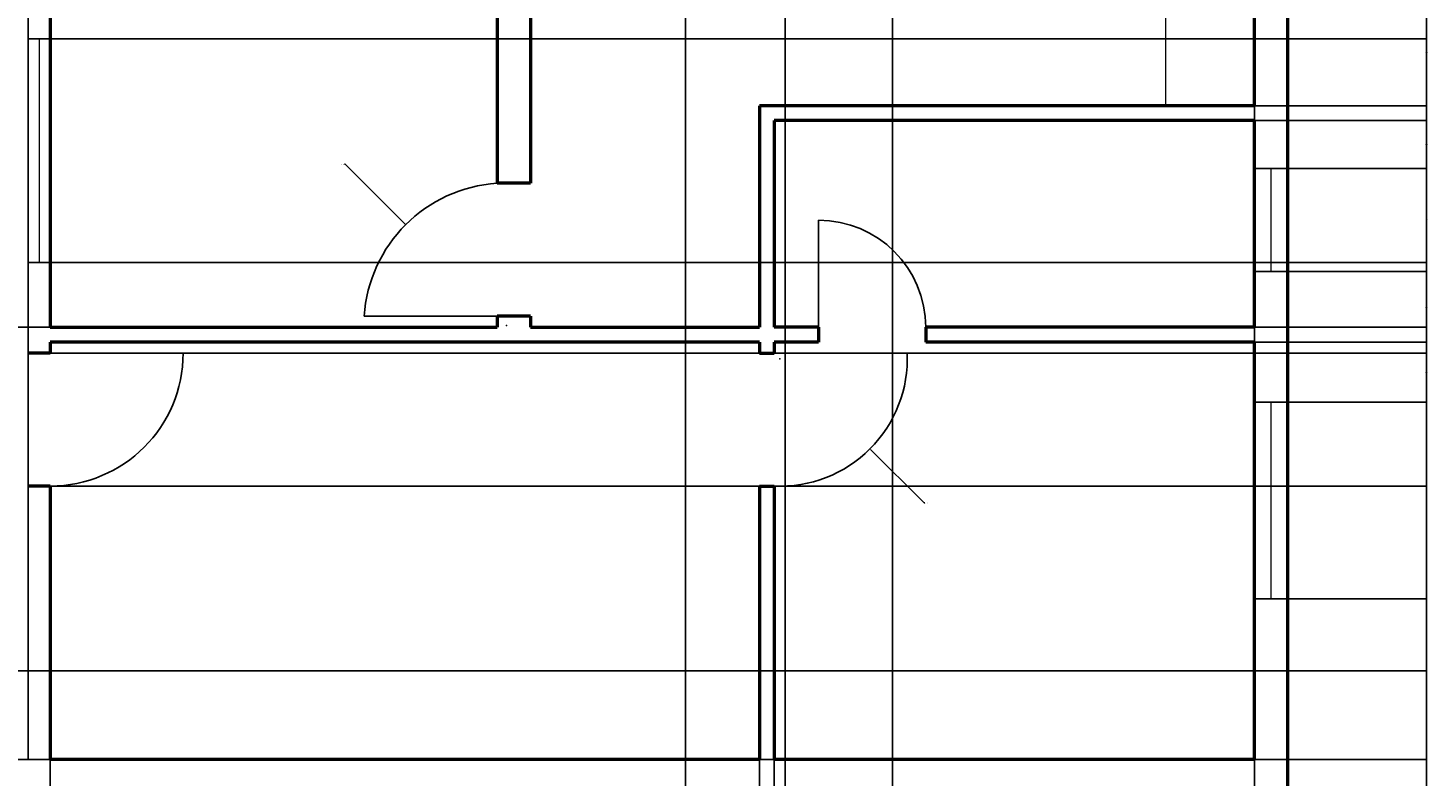
# Model space of a CAD drawing. Units: inches. Extents: x 2479 to 3284, y 2154 to 2936.
# Tile 7 of 8: x 2905 to 3284, y 2538 to 2741. Entities that reach past the tile are written whole.
import ezdxf

# ---------------------------------------------------------------- set-up
doc = ezdxf.new("R2010")
doc.units = ezdxf.units.IN
for name, color, linetype, lineweight in [('A-ANNO-DIMS', 2, 'Continuous', 18), ('A-DOOR', 3, 'Continuous', 25), ('A-FLOR-CASE', 8, 'Continuous', 18), ('A-GLAZ', 4, 'Continuous', 18), ('A-WALL', 7, 'Continuous', 50)]:
    doc.layers.add(name, color=color, linetype=linetype, lineweight=lineweight)
doc.styles.get("Standard").update_dxf_attribs({"font": 'arial.ttf'})
doc.dimstyles.get("Standard").update_dxf_attribs({"dimtxt": 0.18, "dimasz": 0.18, "dimexe": 0.18, "dimexo": 0.0625, "dimgap": 0.09, "dimtad": 0, "dimtih": 1, "dimtoh": 1, "dimdec": 4, "dimzin": 0, "dimdsep": 46, "dimtxsty": 'Standard', "dimcen": 0.09, "dimadec": 0, "dimazin": 0, "dimtfac": 1, "dimtdec": 4, "dimtofl": 0, "dimtmove": 0, "dimatfit": 3, "dimfxl": 1, "dimtolj": 1, "dimtzin": 0, "dimarcsym": 0})

# ---------------------------------------------------------------- blocks, each defined once
blk = doc.blocks.new('DOOR-SWING-29IN')
blk.add_line((29, 0), (0, 0))
blk.add_arc((29, 0), 29, 90, 180)
blk = doc.blocks.new('DOOR-SWING-36IN')
blk.add_line((36, 0), (0, 0))
blk.add_arc((36, 0), 36, 90, 180)
blk = doc.blocks.new('*D10')
at = {"layer": 'A-ANNO-DIMS', "color": 0, "lineweight": -2, "transparency": 16777216}
for p, q in [((3246.27, 2897.74), (3283.99, 2897.74)), ((3283.81, 2897.56), (3283.81, 2715.92)), ((3283.81, 2533.92), (3283.81, 2715.56)), ((3237.27, 2533.74), (3283.99, 2533.74))]:
    blk.add_line(p, q, dxfattribs=at)
at = {"layer": 'A-ANNO-DIMS', "color": 0, "transparency": 16777216}
for points in [[(3283.78, 2897.56), (3283.84, 2897.56), (3283.81, 2897.74)], [(3283.78, 2533.92), (3283.84, 2533.92), (3283.81, 2533.74)]]:
    blk.add_solid(points, dxfattribs=at)
at = {"layer": 'Defpoints', "color": 0, "transparency": 16777216}
for p in [(3246.21, 2897.74), (3283.81, 2897.74), (3237.21, 2533.74)]:
    blk.add_point(p, dxfattribs=at)
at = {"layer": 'A-ANNO-DIMS', "color": 0, "transparency": 16777216, "insert": (3283.81, 2715.74), "char_height": 0.18, "attachment_point": 5}
blk.add_mtext('\\A1;364', dxfattribs=at)
blk = doc.blocks.new('*D11')
at = {"layer": 'A-ANNO-DIMS', "color": 0, "lineweight": -2, "transparency": 16777216}
for p, q in [((2845.21, 2542.8), (2845.21, 2935.52)), ((2845.39, 2935.34), (2874.99, 2935.34)), ((2905.03, 2935.34), (2875.43, 2935.34)), ((2905.21, 2542.8), (2905.21, 2935.52))]:
    blk.add_line(p, q, dxfattribs=at)
at = {"layer": 'A-ANNO-DIMS', "color": 0, "transparency": 16777216}
for points in [[(2845.39, 2935.37), (2845.39, 2935.31), (2845.21, 2935.34)], [(2905.03, 2935.37), (2905.03, 2935.31), (2905.21, 2935.34)]]:
    blk.add_solid(points, dxfattribs=at)
at = {"layer": 'Defpoints', "color": 0, "transparency": 16777216}
for p in [(2905.21, 2935.34), (2845.21, 2542.74), (2905.21, 2542.74)]:
    blk.add_point(p, dxfattribs=at)
at = {"layer": 'A-ANNO-DIMS', "color": 0, "transparency": 16777216, "insert": (2875.21, 2935.34), "char_height": 0.18, "attachment_point": 5}
blk.add_mtext('\\A1;60', dxfattribs=at)
blk = doc.blocks.new('*D20')
at = {"layer": 'A-ANNO-DIMS', "color": 0, "lineweight": -2, "transparency": 16777216}
for p, q in [((2911.27, 2542.74), (3283.99, 2542.74)), ((3283.81, 2542.56), (3283.81, 2538.42)), ((3283.81, 2533.92), (3283.81, 2538.06)), ((2911.27, 2533.74), (3283.99, 2533.74))]:
    blk.add_line(p, q, dxfattribs=at)
at = {"layer": 'A-ANNO-DIMS', "color": 0, "transparency": 16777216}
for points in [[(3283.78, 2542.56), (3283.84, 2542.56), (3283.81, 2542.74)], [(3283.78, 2533.92), (3283.84, 2533.92), (3283.81, 2533.74)]]:
    blk.add_solid(points, dxfattribs=at)
at = {"layer": 'Defpoints', "color": 0, "transparency": 16777216}
for p in [(2911.21, 2542.74), (3283.81, 2542.74), (2911.21, 2533.74)]:
    blk.add_point(p, dxfattribs=at)
at = {"layer": 'A-ANNO-DIMS', "color": 0, "transparency": 16777216, "insert": (3283.81, 2538.24), "char_height": 0.18, "attachment_point": 5}
blk.add_mtext('\\A1;9', dxfattribs=at)
blk = doc.blocks.new('*D21')
at = {"layer": 'A-ANNO-DIMS', "color": 0, "lineweight": -2, "transparency": 16777216}
for p, q in [((2905.27132, 2616.739749), (3283.98882, 2616.739749)), ((3283.80882, 2616.559749), (3283.80882, 2579.919749)), ((3283.80882, 2542.919749), (3283.80882, 2579.559749)), ((2911.27132, 2542.739749), (3283.98882, 2542.739749))]:
    blk.add_line(p, q, dxfattribs=at)
at = {"layer": 'A-ANNO-DIMS', "color": 0, "transparency": 16777216}
for points in [[(3283.77882, 2616.559749), (3283.83882, 2616.559749), (3283.80882, 2616.739749)], [(3283.77882, 2542.919749), (3283.83882, 2542.919749), (3283.80882, 2542.739749)]]:
    blk.add_solid(points, dxfattribs=at)
at = {"layer": 'Defpoints', "color": 0, "transparency": 16777216}
for p in [(2905.20882, 2616.739749), (3283.80882, 2616.739749), (2911.20882, 2542.739749)]:
    blk.add_point(p, dxfattribs=at)
at = {"layer": 'A-ANNO-DIMS', "color": 0, "transparency": 16777216, "insert": (3283.80882, 2579.739749), "char_height": 0.18, "attachment_point": 5}
blk.add_mtext('\\A1;74', dxfattribs=at)
blk = doc.blocks.new('*D22')
at = {"layer": 'A-ANNO-DIMS', "color": 0, "lineweight": -2, "transparency": 16777216}
for p, q in [((2905.27, 2677.32), (3283.99, 2677.32)), ((3283.81, 2677.14), (3283.81, 2665.21)), ((3283.81, 2652.92), (3283.81, 2664.85)), ((2905.27, 2652.74), (3283.99, 2652.74))]:
    blk.add_line(p, q, dxfattribs=at)
at = {"layer": 'A-ANNO-DIMS', "color": 0, "transparency": 16777216}
for points in [[(3283.78, 2677.14), (3283.84, 2677.14), (3283.81, 2677.32)], [(3283.78, 2652.92), (3283.84, 2652.92), (3283.81, 2652.74)]]:
    blk.add_solid(points, dxfattribs=at)
at = {"layer": 'Defpoints', "color": 0, "transparency": 16777216}
for p in [(2905.21, 2677.32), (3283.81, 2677.32), (2905.21, 2652.74)]:
    blk.add_point(p, dxfattribs=at)
at = {"layer": 'A-ANNO-DIMS', "color": 0, "transparency": 16777216, "insert": (3283.81, 2665.03), "char_height": 0.18, "attachment_point": 5}
blk.add_mtext('\\A1;24.575', dxfattribs=at)
blk = doc.blocks.new('*D23')
at = {"layer": 'A-ANNO-DIMS', "color": 0, "lineweight": -2, "transparency": 16777216}
for p, q in [((2905.27, 2737.84), (3283.99, 2737.84)), ((3283.81, 2737.66), (3283.81, 2707.76)), ((3283.81, 2677.5), (3283.81, 2707.39)), ((2905.27, 2677.32), (3283.99, 2677.32))]:
    blk.add_line(p, q, dxfattribs=at)
at = {"layer": 'A-ANNO-DIMS', "color": 0, "transparency": 16777216}
for points in [[(3283.78, 2737.66), (3283.84, 2737.66), (3283.81, 2737.84)], [(3283.78, 2677.5), (3283.84, 2677.5), (3283.81, 2677.32)]]:
    blk.add_solid(points, dxfattribs=at)
at = {"layer": 'Defpoints', "color": 0, "transparency": 16777216}
for p in [(2905.21, 2737.84), (3283.81, 2737.84), (2905.21, 2677.32)]:
    blk.add_point(p, dxfattribs=at)
at = {"layer": 'A-ANNO-DIMS', "color": 0, "transparency": 16777216, "insert": (3283.81, 2707.58), "char_height": 0.18, "attachment_point": 5}
blk.add_mtext('\\A1;60.52', dxfattribs=at)
blk = doc.blocks.new('*D61')
at = {"layer": 'A-ANNO-DIMS', "color": 0, "lineweight": -2, "transparency": 16777216}
for p, q in [((2595.27, 2566.74), (3283.99, 2566.74)), ((3283.81, 2566.56), (3283.81, 2554.92)), ((3283.81, 2542.92), (3283.81, 2554.56)), ((2595.27, 2542.74), (3283.99, 2542.74))]:
    blk.add_line(p, q, dxfattribs=at)
at = {"layer": 'A-ANNO-DIMS', "color": 0, "transparency": 16777216}
for points in [[(3283.78, 2566.56), (3283.84, 2566.56), (3283.81, 2566.74)], [(3283.78, 2542.92), (3283.84, 2542.92), (3283.81, 2542.74)]]:
    blk.add_solid(points, dxfattribs=at)
at = {"layer": 'Defpoints', "color": 0, "transparency": 16777216}
for p in [(2595.21, 2566.74), (3283.81, 2566.74), (2595.21, 2542.74)]:
    blk.add_point(p, dxfattribs=at)
at = {"layer": 'A-ANNO-DIMS', "color": 0, "transparency": 16777216, "insert": (3283.81, 2554.74), "char_height": 0.18, "attachment_point": 5}
blk.add_mtext('\\A1;24', dxfattribs=at)
blk = doc.blocks.new('*D74')
at = {"layer": 'A-ANNO-DIMS', "color": 0, "lineweight": -2, "transparency": 16777216}
for p, q in [((3237.27, 2586.18), (3283.99, 2586.18)), ((3283.81, 2586), (3283.81, 2564.64)), ((3283.81, 2542.92), (3283.81, 2564.28)), ((3237.27, 2542.74), (3283.99, 2542.74))]:
    blk.add_line(p, q, dxfattribs=at)
at = {"layer": 'A-ANNO-DIMS', "color": 0, "transparency": 16777216}
for points in [[(3283.78, 2586), (3283.84, 2586), (3283.81, 2586.18)], [(3283.78, 2542.92), (3283.84, 2542.92), (3283.81, 2542.74)]]:
    blk.add_solid(points, dxfattribs=at)
at = {"layer": 'Defpoints', "color": 0, "transparency": 16777216}
for p in [(3237.21, 2586.18), (3283.81, 2586.18), (3237.21, 2542.74)]:
    blk.add_point(p, dxfattribs=at)
at = {"layer": 'A-ANNO-DIMS', "color": 0, "transparency": 16777216, "insert": (3283.81, 2564.46), "char_height": 0.18, "attachment_point": 5}
blk.add_mtext('\\A1;43.44', dxfattribs=at)
blk = doc.blocks.new('*D75')
at = {"layer": 'A-ANNO-DIMS', "color": 0, "lineweight": -2, "transparency": 16777216}
for p, q in [((3237.27, 2639.44), (3283.99, 2639.44)), ((3283.81, 2639.26), (3283.81, 2612.99)), ((3283.81, 2586.36), (3283.81, 2612.62)), ((3237.27, 2586.18), (3283.99, 2586.18))]:
    blk.add_line(p, q, dxfattribs=at)
at = {"layer": 'A-ANNO-DIMS', "color": 0, "transparency": 16777216}
for points in [[(3283.78, 2639.26), (3283.84, 2639.26), (3283.81, 2639.44)], [(3283.78, 2586.36), (3283.84, 2586.36), (3283.81, 2586.18)]]:
    blk.add_solid(points, dxfattribs=at)
at = {"layer": 'Defpoints', "color": 0, "transparency": 16777216}
for p in [(3237.21, 2639.44), (3283.81, 2639.44), (3237.21, 2586.18)]:
    blk.add_point(p, dxfattribs=at)
at = {"layer": 'A-ANNO-DIMS', "color": 0, "transparency": 16777216, "insert": (3283.81, 2612.81), "char_height": 0.18, "attachment_point": 5}
blk.add_mtext('\\A1;53.26', dxfattribs=at)
blk = doc.blocks.new('*D76')
at = {"layer": 'A-ANNO-DIMS', "color": 0, "lineweight": -2, "transparency": 16777216}
for p, q in [((3237.27, 2655.74), (3283.99, 2655.74)), ((3283.81, 2655.56), (3283.81, 2647.77)), ((3283.81, 2639.62), (3283.81, 2647.41)), ((3237.27, 2639.44), (3283.99, 2639.44))]:
    blk.add_line(p, q, dxfattribs=at)
at = {"layer": 'A-ANNO-DIMS', "color": 0, "transparency": 16777216}
for points in [[(3283.78, 2655.56), (3283.84, 2655.56), (3283.81, 2655.74)], [(3283.78, 2639.62), (3283.84, 2639.62), (3283.81, 2639.44)]]:
    blk.add_solid(points, dxfattribs=at)
at = {"layer": 'Defpoints', "color": 0, "transparency": 16777216}
for p in [(3237.21, 2655.74), (3283.81, 2655.74), (3237.21, 2639.44)]:
    blk.add_point(p, dxfattribs=at)
at = {"layer": 'A-ANNO-DIMS', "color": 0, "transparency": 16777216, "insert": (3283.81, 2647.59), "char_height": 0.18, "attachment_point": 5}
blk.add_mtext('\\A1;16.305', dxfattribs=at)
blk = doc.blocks.new('*D77')
at = {"layer": 'A-ANNO-DIMS', "color": 0, "lineweight": -2, "transparency": 16777216}
for p, q in [((3237.27, 2674.89), (3283.99, 2674.89)), ((3283.81, 2674.71), (3283.81, 2667.5)), ((3283.81, 2659.92), (3283.81, 2667.13)), ((3237.27, 2659.74), (3283.99, 2659.74))]:
    blk.add_line(p, q, dxfattribs=at)
at = {"layer": 'A-ANNO-DIMS', "color": 0, "transparency": 16777216}
for points in [[(3283.78, 2674.71), (3283.84, 2674.71), (3283.81, 2674.89)], [(3283.78, 2659.92), (3283.84, 2659.92), (3283.81, 2659.74)]]:
    blk.add_solid(points, dxfattribs=at)
at = {"layer": 'Defpoints', "color": 0, "transparency": 16777216}
for p in [(3237.21, 2674.89), (3283.81, 2674.89), (3237.21, 2659.74)]:
    blk.add_point(p, dxfattribs=at)
at = {"layer": 'A-ANNO-DIMS', "color": 0, "transparency": 16777216, "insert": (3283.81, 2667.31), "char_height": 0.18, "attachment_point": 5}
blk.add_mtext('\\A1;15.15', dxfattribs=at)
blk = doc.blocks.new('*D78')
at = {"layer": 'A-ANNO-DIMS', "color": 0, "lineweight": -2, "transparency": 16777216}
for p, q in [((3237.27, 2702.73), (3283.99, 2702.73)), ((3283.81, 2702.55), (3283.81, 2688.99)), ((3283.81, 2675.07), (3283.81, 2688.63)), ((3237.27, 2674.89), (3283.99, 2674.89))]:
    blk.add_line(p, q, dxfattribs=at)
at = {"layer": 'A-ANNO-DIMS', "color": 0, "transparency": 16777216}
for points in [[(3283.78, 2702.55), (3283.84, 2702.55), (3283.81, 2702.73)], [(3283.78, 2675.07), (3283.84, 2675.07), (3283.81, 2674.89)]]:
    blk.add_solid(points, dxfattribs=at)
at = {"layer": 'Defpoints', "color": 0, "transparency": 16777216}
for p in [(3237.21, 2702.73), (3283.81, 2702.73), (3237.21, 2674.89)]:
    blk.add_point(p, dxfattribs=at)
at = {"layer": 'A-ANNO-DIMS', "color": 0, "transparency": 16777216, "insert": (3283.81, 2688.81), "char_height": 0.18, "attachment_point": 5}
blk.add_mtext('\\A1;27.837', dxfattribs=at)
blk = doc.blocks.new('*D79')
at = {"layer": 'A-ANNO-DIMS', "color": 0, "lineweight": -2, "transparency": 16777216}
for p, q in [((3237.27, 2715.74), (3283.99, 2715.74)), ((3283.81, 2715.56), (3283.81, 2709.42)), ((3283.81, 2702.91), (3283.81, 2709.05)), ((3237.27, 2702.73), (3283.99, 2702.73))]:
    blk.add_line(p, q, dxfattribs=at)
at = {"layer": 'A-ANNO-DIMS', "color": 0, "transparency": 16777216}
for points in [[(3283.78, 2715.56), (3283.84, 2715.56), (3283.81, 2715.74)], [(3283.78, 2702.91), (3283.84, 2702.91), (3283.81, 2702.73)]]:
    blk.add_solid(points, dxfattribs=at)
at = {"layer": 'Defpoints', "color": 0, "transparency": 16777216}
for p in [(3237.21, 2715.74), (3283.81, 2715.74), (3237.21, 2702.73)]:
    blk.add_point(p, dxfattribs=at)
at = {"layer": 'A-ANNO-DIMS', "color": 0, "transparency": 16777216, "insert": (3283.81, 2709.23), "char_height": 0.18, "attachment_point": 5}
blk.add_mtext('\\A1;13.013', dxfattribs=at)
blk = doc.blocks.new('*D80')
at = {"layer": 'A-ANNO-DIMS', "color": 0, "lineweight": -2, "transparency": 16777216}
for p, q in [((3237.27, 2748.61), (3283.99, 2748.61)), ((3283.81, 2748.43), (3283.81, 2734.36)), ((3283.81, 2719.92), (3283.81, 2733.99)), ((3237.27, 2719.74), (3283.99, 2719.74))]:
    blk.add_line(p, q, dxfattribs=at)
at = {"layer": 'A-ANNO-DIMS', "color": 0, "transparency": 16777216}
for points in [[(3283.78, 2748.43), (3283.84, 2748.43), (3283.81, 2748.61)], [(3283.78, 2719.92), (3283.84, 2719.92), (3283.81, 2719.74)]]:
    blk.add_solid(points, dxfattribs=at)
at = {"layer": 'Defpoints', "color": 0, "transparency": 16777216}
for p in [(3237.21, 2748.61), (3283.81, 2748.61), (3237.21, 2719.74)]:
    blk.add_point(p, dxfattribs=at)
at = {"layer": 'A-ANNO-DIMS', "color": 0, "transparency": 16777216, "insert": (3283.81, 2734.18), "char_height": 0.18, "attachment_point": 5}
blk.add_mtext('\\A1;28.874', dxfattribs=at)
blk = doc.blocks.new('*D86')
at = {"layer": 'A-ANNO-DIMS', "color": 0, "lineweight": -2, "transparency": 16777216}
for p, q in [((3041.15, 2770.74), (2479.43, 2770.74)), ((2479.61, 2770.56), (2479.61, 2715.42)), ((2479.61, 2659.92), (2479.61, 2715.06)), ((2911.15, 2659.74), (2479.43, 2659.74))]:
    blk.add_line(p, q, dxfattribs=at)
at = {"layer": 'A-ANNO-DIMS', "color": 0, "transparency": 16777216}
for points in [[(2479.58, 2770.56), (2479.64, 2770.56), (2479.61, 2770.74)], [(2479.58, 2659.92), (2479.64, 2659.92), (2479.61, 2659.74)]]:
    blk.add_solid(points, dxfattribs=at)
at = {"layer": 'Defpoints', "color": 0, "transparency": 16777216}
for p in [(2479.61, 2770.74), (3041.21, 2770.74), (2911.21, 2659.74)]:
    blk.add_point(p, dxfattribs=at)
at = {"layer": 'A-ANNO-DIMS', "color": 0, "transparency": 16777216, "insert": (2479.61, 2715.24), "char_height": 0.18, "attachment_point": 5}
blk.add_mtext('\\A1;111', dxfattribs=at)
blk = doc.blocks.new('*D87')
at = {"layer": 'A-ANNO-DIMS', "color": 0, "lineweight": -2, "transparency": 16777216}
for p, q in [((2911.21, 2542.68), (2911.21, 2153.96)), ((3103.21, 2542.68), (3103.21, 2153.96)), ((2911.39, 2154.14), (3006.93, 2154.14)), ((3103.03, 2154.14), (3007.49, 2154.14))]:
    blk.add_line(p, q, dxfattribs=at)
at = {"layer": 'A-ANNO-DIMS', "color": 0, "transparency": 16777216}
for points in [[(2911.39, 2154.17), (2911.39, 2154.11), (2911.21, 2154.14)], [(3103.03, 2154.17), (3103.03, 2154.11), (3103.21, 2154.14)]]:
    blk.add_solid(points, dxfattribs=at)
at = {"layer": 'Defpoints', "color": 0, "transparency": 16777216}
for p in [(2911.21, 2542.74), (3103.21, 2542.74), (3103.21, 2154.14)]:
    blk.add_point(p, dxfattribs=at)
at = {"layer": 'A-ANNO-DIMS', "color": 0, "transparency": 16777216, "insert": (3007.21, 2154.14), "char_height": 0.18, "attachment_point": 5}
blk.add_mtext('\\A1;192', dxfattribs=at)
blk = doc.blocks.new('*D88')
at = {"layer": 'A-ANNO-DIMS', "color": 0, "lineweight": -2, "transparency": 16777216}
for p, q in [((3107.21, 2542.68), (3107.21, 2153.96)), ((3237.21, 2542.68), (3237.21, 2153.96)), ((3107.39, 2154.14), (3171.93, 2154.14)), ((3237.03, 2154.14), (3172.49, 2154.14))]:
    blk.add_line(p, q, dxfattribs=at)
at = {"layer": 'A-ANNO-DIMS', "color": 0, "transparency": 16777216}
for points in [[(3107.39, 2154.17), (3107.39, 2154.11), (3107.21, 2154.14)], [(3237.03, 2154.17), (3237.03, 2154.11), (3237.21, 2154.14)]]:
    blk.add_solid(points, dxfattribs=at)
at = {"layer": 'Defpoints', "color": 0, "transparency": 16777216}
for p in [(3107.21, 2542.74), (3237.21, 2542.74), (3237.21, 2154.14)]:
    blk.add_point(p, dxfattribs=at)
at = {"layer": 'A-ANNO-DIMS', "color": 0, "transparency": 16777216, "insert": (3172.21, 2154.14), "char_height": 0.18, "attachment_point": 5}
blk.add_mtext('\\A1;130', dxfattribs=at)
blk = doc.blocks.new('*D131')
at = {"layer": 'A-ANNO-DIMS', "color": 0, "lineweight": -2, "transparency": 16777216}
for p, q in [((3083.21, 2407.8), (3083.21, 2935.52)), ((3083.39, 2935.34), (3096.49, 2935.34)), ((3110.03, 2935.34), (3096.93, 2935.34)), ((3110.21, 2407.8), (3110.21, 2935.52))]:
    blk.add_line(p, q, dxfattribs=at)
at = {"layer": 'A-ANNO-DIMS', "color": 0, "transparency": 16777216}
for points in [[(3083.39, 2935.37), (3083.39, 2935.31), (3083.21, 2935.34)], [(3110.03, 2935.37), (3110.03, 2935.31), (3110.21, 2935.34)]]:
    blk.add_solid(points, dxfattribs=at)
at = {"layer": 'Defpoints', "color": 0, "transparency": 16777216}
for p in [(3110.21, 2935.34), (3083.21, 2407.74), (3110.21, 2407.74)]:
    blk.add_point(p, dxfattribs=at)
at = {"layer": 'A-ANNO-DIMS', "color": 0, "transparency": 16777216, "insert": (3096.71, 2935.34), "char_height": 0.18, "attachment_point": 5}
blk.add_mtext('\\A1;27', dxfattribs=at)
blk = doc.blocks.new('*D132')
at = {"layer": 'A-ANNO-DIMS', "color": 0, "lineweight": -2, "transparency": 16777216}
for p, q in [((3139.21, 2407.8), (3139.21, 2935.52)), ((3139.39, 2935.34), (3187.99, 2935.34)), ((3237.03, 2935.34), (3188.43, 2935.34)), ((3237.21, 2407.8), (3237.21, 2935.52))]:
    blk.add_line(p, q, dxfattribs=at)
at = {"layer": 'A-ANNO-DIMS', "color": 0, "transparency": 16777216}
for points in [[(3139.39, 2935.37), (3139.39, 2935.31), (3139.21, 2935.34)], [(3237.03, 2935.37), (3237.03, 2935.31), (3237.21, 2935.34)]]:
    blk.add_solid(points, dxfattribs=at)
at = {"layer": 'Defpoints', "color": 0, "transparency": 16777216}
for p in [(3237.21, 2935.34), (3139.21, 2407.74), (3237.21, 2407.74)]:
    blk.add_point(p, dxfattribs=at)
at = {"layer": 'A-ANNO-DIMS', "color": 0, "transparency": 16777216, "insert": (3188.21, 2935.34), "char_height": 0.18, "attachment_point": 5}
blk.add_mtext('\\A1;98', dxfattribs=at)
blk = doc.blocks.new('*D133')
at = {"layer": 'A-ANNO-DIMS', "color": 0, "lineweight": -2, "transparency": 16777216}
for p, q in [((2990.87, 2703.89), (2991.05, 2703.89)), ((2991.05, 2703.89), (3007.31, 2687.64)), ((3034.64, 2660.22), (3034.82, 2660.22)), ((3034.73, 2660.13), (3034.73, 2660.31))]:
    blk.add_line(p, q, dxfattribs=at)
at = {"layer": 'A-ANNO-DIMS', "color": 0, "transparency": 16777216}
blk.add_solid([(3007.33, 2687.66), (3007.29, 2687.62), (3007.43, 2687.52)], dxfattribs=at)
at = {"layer": 'Defpoints', "color": 0, "transparency": 16777216}
for p in [(3007.43, 2687.52), (3034.73, 2660.22)]:
    blk.add_point(p, dxfattribs=at)
at = {"layer": 'A-ANNO-DIMS', "color": 0, "transparency": 16777216, "insert": (2990.32, 2703.89), "char_height": 0.18, "attachment_point": 5}
blk.add_mtext('\\A1;R38.605', dxfattribs=at)
blk = doc.blocks.new('*D134')
at = {"layer": 'A-ANNO-DIMS', "color": 0, "lineweight": -2, "transparency": 16777216}
for p, q in [((3108.62, 2651.24), (3108.8, 2651.24)), ((3108.71, 2651.15), (3108.71, 2651.33)), ((3147.78, 2612.17), (3133.26, 2626.69)), ((3147.96, 2612.17), (3147.78, 2612.17))]:
    blk.add_line(p, q, dxfattribs=at)
at = {"layer": 'A-ANNO-DIMS', "color": 0, "transparency": 16777216}
blk.add_solid([(3133.28, 2626.71), (3133.23, 2626.67), (3133.13, 2626.82)], dxfattribs=at)
at = {"layer": 'Defpoints', "color": 0, "transparency": 16777216}
for p in [(3108.71, 2651.24), (3133.13, 2626.82)]:
    blk.add_point(p, dxfattribs=at)
at = {"layer": 'A-ANNO-DIMS', "color": 0, "transparency": 16777216, "insert": (3148.44, 2612.17), "char_height": 0.18, "attachment_point": 5}
blk.add_mtext('\\A1;R34.53', dxfattribs=at)

msp = doc.modelspace()

# ---------------------------------------------------------------- linework, layer by layer
at = {"layer": 'A-DOOR'}
for p, q in [((3032.2088, 2662.7397), (2996.2088, 2662.7397)), ((3107.2088, 2652.7397), (3143.2088, 2652.7397))]:
    msp.add_line(p, q, dxfattribs=at)
for centre, radius, start, end in [((3034.7318, 2660.2168), 38.6055, 93.747096, 176.252904), ((3108.7128, 2651.2357), 34.5288, 267.50349, 2.49651)]:
    msp.add_arc(centre, radius, start, end, dxfattribs=at)
at = {"layer": 'A-FLOR-CASE'}
msp.add_line((3213.2088, 2719.7397), (3213.2088, 2809.7397), dxfattribs=at)
at = {"layer": 'A-GLAZ'}
for p, q in [((2911.2088, 2737.8354), (2905.2088, 2737.8354)), ((2908.2088, 2737.8354), (2908.2088, 2677.3151)), ((3237.2088, 2702.7268), (3246.2088, 2702.7268)), ((3241.7088, 2674.8898), (3241.7088, 2702.7268)), ((2911.2088, 2677.3151), (2905.2088, 2677.3151)), ((3237.2088, 2674.8898), (3246.2088, 2674.8898)), ((3237.2088, 2639.4351), (3246.2088, 2639.4351)), ((3241.7088, 2586.1783), (3241.7088, 2639.4351)), ((3237.2088, 2586.1783), (3246.2088, 2586.1783))]:
    msp.add_line(p, q, dxfattribs=at)
at = {"layer": 'A-WALL'}
for p, q in [((3246.2088, 2191.7397), (3246.2088, 2897.7397)), ((2911.2088, 2845.7397), (2911.2088, 2659.7397)), ((3237.2088, 2719.7397), (3237.2088, 2833.7397)), ((3032.2088, 2777.7397), (3032.2088, 2698.7397)), ((3041.2088, 2770.7397), (3041.2088, 2698.7397)), ((3107.2088, 2719.7397), (3103.2088, 2719.7397)), ((3103.2088, 2719.7397), (3103.2088, 2659.7397)), ((3237.2088, 2719.7397), (3107.2088, 2719.7397)), ((3237.2088, 2715.7397), (3107.2088, 2715.7397)), ((3107.2088, 2715.7397), (3107.2088, 2659.7397)), ((3237.2088, 2659.7397), (3237.2088, 2715.7397)), ((3041.2088, 2698.7397), (3032.2088, 2698.7397)), ((3041.2088, 2662.7397), (3032.2088, 2662.7397)), ((3032.2088, 2662.7397), (3032.2088, 2659.7397)), ((3041.2088, 2662.7397), (3041.2088, 2659.7397)), ((2911.2088, 2659.7397), (3032.2088, 2659.7397)), ((3041.2088, 2659.7397), (3103.2088, 2659.7397)), ((3119.2088, 2659.7397), (3107.2088, 2659.7397)), ((3119.2088, 2659.7397), (3119.2088, 2655.7397)), ((3237.2088, 2659.7397), (3148.2088, 2659.7397)), ((3148.2088, 2659.7397), (3148.2088, 2655.7397)), ((3103.2088, 2655.7397), (2911.2088, 2655.7397)), ((2911.2088, 2655.7397), (2911.2088, 2652.7397)), ((3103.2088, 2655.7397), (3103.2088, 2652.7397)), ((3107.2088, 2655.7397), (3107.2088, 2652.7397)), ((3119.2088, 2655.7397), (3107.2088, 2655.7397)), ((3237.2088, 2655.7397), (3148.2088, 2655.7397)), ((3237.2088, 2542.7397), (3237.2088, 2655.7397)), ((2911.2088, 2652.7397), (2905.2088, 2652.7397)), ((3103.2088, 2652.7397), (3107.2088, 2652.7397)), ((2911.2088, 2616.7397), (2905.2088, 2616.7397)), ((2911.2088, 2616.7397), (2911.2088, 2542.7397)), ((3103.2088, 2616.7397), (3107.2088, 2616.7397)), ((3103.2088, 2616.7397), (3103.2088, 2542.7397)), ((3107.2088, 2616.7397), (3107.2088, 2542.7397)), ((3103.2088, 2542.7397), (2911.2088, 2542.7397)), ((3237.2088, 2542.7397), (3107.2088, 2542.7397))]:
    msp.add_line(p, q, dxfattribs=at)

# ---------------------------------------------------------------- block references
at = {"layer": 'A-DOOR'}
for name, p, rotation in [('DOOR-SWING-29IN', (3119.2088, 2688.7397), 270.0000000000005), ('DOOR-SWING-36IN', (2947.2088, 2652.7397), 180)]:
    msp.add_blockref(name, p, dxfattribs=dict(at, rotation=rotation))

# ---------------------------------------------------------------- dimensions: what is measured, and where the dimension line sits
at = {"layer": 'A-ANNO-DIMS'}
for base, p1, p2, picture, middle in [((2905.2088, 2935.3397), (2845.2088, 2542.7397), (2905.2088, 2542.7397), '*D11', (2875.2088, 2935.3397)), ((3110.2088, 2935.3397), (3083.2088, 2407.7397), (3110.2088, 2407.7397), '*D131', (3096.7088, 2935.3397)), ((3237.2088, 2935.3397), (3139.2088, 2407.7397), (3237.2088, 2407.7397), '*D132', (3188.2088, 2935.3397)), ((3103.2088, 2154.1397), (2911.2088, 2542.7397), (3103.2088, 2542.7397), '*D87', (3007.2088, 2154.1397)), ((3237.2088, 2154.1397), (3107.2088, 2542.7397), (3237.2088, 2542.7397), '*D88', (3172.2088, 2154.1397))]:
    dim = msp.add_linear_dim(base=base, p1=p1, p2=p2, dimstyle='Standard', override={"dimdec": 0, "dimlfac": 1, "dimrnd": 0, "dimzin": 0, "dimdsep": 46, "dimlunit": 2}, dxfattribs=at)
    dim.commit()
    dim.dimension.update_dxf_attribs({"geometry": picture, "text_midpoint": middle})
for base, p1, p2, override, picture, middle in [((3283.8088, 2897.7397), (3237.2088, 2533.7397), (3246.2088, 2897.7397), {"dimdec": 0, "dimlfac": 1, "dimrnd": 0, "dimzin": 0, "dimdsep": 46, "dimlunit": 2}, '*D10', (3283.8088, 2715.7397)), ((2479.6088, 2770.7397), (2911.2088, 2659.7397), (3041.2088, 2770.7397), {"dimdec": 0, "dimlfac": 1, "dimrnd": 0, "dimzin": 0, "dimdsep": 46, "dimlunit": 2}, '*D86', (2479.6088, 2715.2397)), ((3283.8088, 2748.6135), (3237.2088, 2719.7397), (3237.2088, 2748.6135), {"dimdec": 3, "dimlfac": 1, "dimrnd": 0, "dimzin": 0, "dimdsep": 46, "dimlunit": 2}, '*D80', (3283.8088, 2734.1766)), ((3283.8088, 2737.8354), (2905.2088, 2677.3151), (2905.2088, 2737.8354), {"dimdec": 2, "dimlfac": 1, "dimrnd": 0, "dimzin": 0, "dimdsep": 46, "dimlunit": 2}, '*D23', (3283.8088, 2707.5753)), ((3283.8088, 2715.7397), (3237.2088, 2702.7268), (3237.2088, 2715.7397), {"dimdec": 3, "dimlfac": 1, "dimrnd": 0, "dimzin": 0, "dimdsep": 46, "dimlunit": 2}, '*D79', (3283.8088, 2709.2333)), ((3283.8088, 2702.7268), (3237.2088, 2674.8898), (3237.2088, 2702.7268), {"dimdec": 3, "dimlfac": 1, "dimrnd": 0, "dimzin": 0, "dimdsep": 46, "dimlunit": 2}, '*D78', (3283.8088, 2688.8083)), ((3283.8088, 2677.3151), (2905.2088, 2652.7397), (2905.2088, 2677.3151), {"dimdec": 3, "dimlfac": 1, "dimrnd": 0, "dimzin": 0, "dimdsep": 46, "dimlunit": 2}, '*D22', (3283.8088, 2665.0274)), ((3283.8088, 2674.8898), (3237.2088, 2659.7397), (3237.2088, 2674.8898), {"dimdec": 2, "dimlfac": 1, "dimrnd": 0, "dimzin": 0, "dimdsep": 46, "dimlunit": 2}, '*D77', (3283.8088, 2667.3148)), ((3283.8088, 2655.7397), (3237.2088, 2639.4351), (3237.2088, 2655.7397), {"dimdec": 3, "dimlfac": 1, "dimrnd": 0, "dimzin": 0, "dimdsep": 46, "dimlunit": 2}, '*D76', (3283.8088, 2647.5874)), ((3283.8088, 2639.4351), (3237.2088, 2586.1783), (3237.2088, 2639.4351), {"dimdec": 2, "dimlfac": 1, "dimrnd": 0, "dimzin": 0, "dimdsep": 46, "dimlunit": 2}, '*D75', (3283.8088, 2612.8067)), ((3283.8088, 2616.7397), (2911.2088, 2542.7397), (2905.2088, 2616.7397), {"dimdec": 0, "dimlfac": 1, "dimrnd": 0, "dimzin": 0, "dimdsep": 46, "dimlunit": 2}, '*D21', (3283.8088, 2579.7397)), ((3283.8088, 2586.1783), (3237.2088, 2542.7397), (3237.2088, 2586.1783), {"dimdec": 2, "dimlfac": 1, "dimrnd": 0, "dimzin": 0, "dimdsep": 46, "dimlunit": 2}, '*D74', (3283.8088, 2564.459)), ((3283.8088, 2566.7397), (2595.2088, 2542.7397), (2595.2088, 2566.7397), {"dimdec": 0, "dimlfac": 1, "dimrnd": 0, "dimzin": 0, "dimdsep": 46, "dimlunit": 2}, '*D61', (3283.8088, 2554.7397)), ((3283.8088, 2542.7397), (2911.2088, 2533.7397), (2911.2088, 2542.7397), {"dimdec": 0, "dimlfac": 1, "dimrnd": 0, "dimzin": 0, "dimdsep": 46, "dimlunit": 2}, '*D20', (3283.8088, 2538.2397))]:
    dim = msp.add_linear_dim(base=base, p1=p1, p2=p2, angle=90, dimstyle='Standard', override=override, dxfattribs=at)
    dim.commit()
    dim.dimension.update_dxf_attribs({"geometry": picture, "text_midpoint": middle})
for center, mpoint, override, picture, middle in [((3034.7318, 2660.2168), (3007.4338, 2687.5152), {"dimdec": 3, "dimlfac": 1, "dimrnd": 0, "dimzin": 0, "dimdsep": 46, "dimlunit": 2}, '*D133', (2990.3246, 2703.8943)), ((3108.7128, 2651.2357), (3133.1281, 2626.8199), {"dimdec": 2, "dimlfac": 1, "dimrnd": 0, "dimzin": 0, "dimdsep": 46, "dimlunit": 2}, '*D134', (3148.437, 2612.1705))]:
    dim = msp.add_radius_dim(center=center, mpoint=mpoint, dimstyle='Standard', override=override, dxfattribs=at)
    dim.commit()
    dim.dimension.update_dxf_attribs({"geometry": picture, "text_midpoint": middle, "dimtype": 164})

doc.saveas('drawing.dxf')
